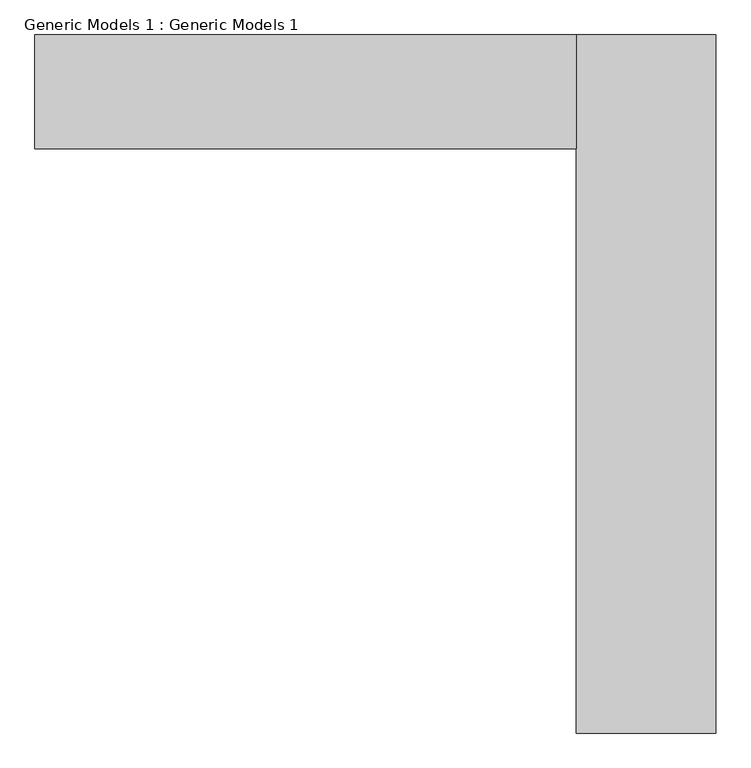
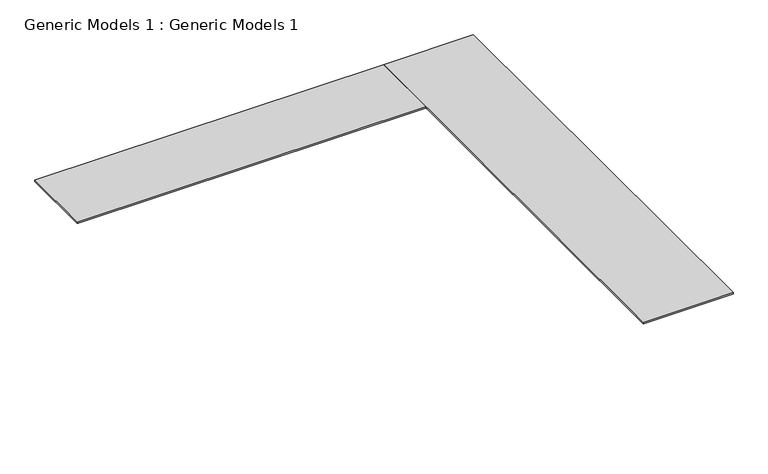
"""IFC4 building model written with IfcOpenShell, lengths in millimetres: proxy geometry, Generic Models 1 : Generic Models 1."""

from ifc_helpers import new_model, si_unit, frame, origin, place, context, project, spatial, polyline, outline, extrude, source, transform, mapped, element, save


def generic_models_1_generic_models_1_85262742(model_context):
    return source(origin(), model_context, "Body", "SweptSolid", [
        extrude(outline(polyline([(11042.65, 14886.6878923), (-5498.4090453, 14886.6878923), (-5498.4090453, 18362.4927525), (11042.65, 18362.4927525), (11042.65, 14886.6878923)])), frame((0.0, 0.0, -76.2), z_axis=(0.0, 0.0, 1.0), x_axis=(1.0, 0.0, 0.0)), (0.0, 0.0, 1.0), 76.2),
        extrude(outline(polyline([(15309.85, 18362.4927525), (15309.85, -2973.5072475), (11042.65, -2973.5072475), (11042.65, 18362.4927525), (15309.85, 18362.4927525)])), frame((0.0, 0.0, -76.2), z_axis=(0.0, 0.0, 1.0), x_axis=(1.0, 0.0, 0.0)), (0.0, 0.0, 1.0), 76.2),
    ])


if __name__ == "__main__":
    model = new_model("IFC4")
    model_context = context("Model", 3, world=origin())
    ifc_project = project(units=[si_unit("LENGTHUNIT", "METRE", prefix="MILLI")], contexts=[model_context])
    site = spatial("IfcSite", under=ifc_project)
    building = spatial("IfcBuilding", under=site)
    placement = place(None, origin())
    generic_models_1_generic_models_1_shape = generic_models_1_generic_models_1_85262742(model_context)
    element("IfcBuildingElementProxy", 1, Name="Generic Models 1 : Generic Models 1", ObjectType="Generic Models 1 : Generic Models 1", at=placement, inside=building, context=model_context, shape_type="MappedRepresentation", body=[
        mapped(generic_models_1_generic_models_1_shape, transform((0.0, 0.0, 0.0), x_axis=(1.0, 0.0, 0.0), y_axis=(0.0, 1.0, 0.0), z_axis=(0.0, 0.0, 1.0))),
    ])
    save(model, "model.ifc")
